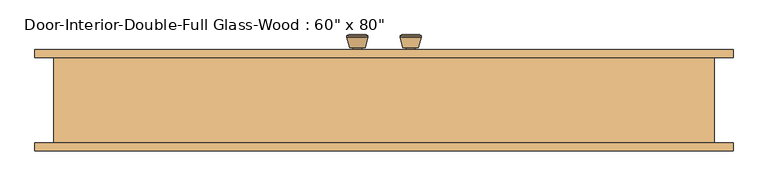
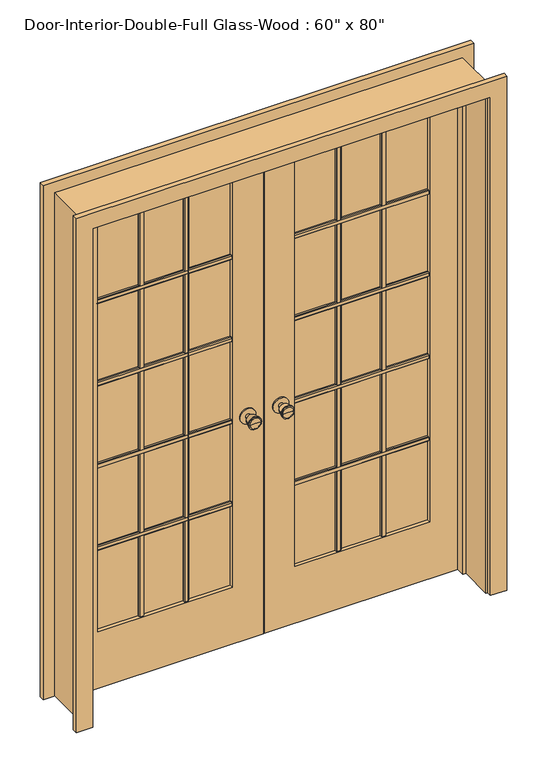
"""IFC4 building model written with IfcOpenShell, lengths in millimetres: door geometry."""

from ifc_helpers import new_model, si_unit, point, frame, frame_2d, origin, place, context, project, spatial, polyline, circle_curve, trimmed, segment, composite_curve, outline, extrude, faceted_brep, source, transform, mapped, element, save
from ifc_brep_helpers import plane_surface, cylinder_surface, revolved_surface, advanced_brep


def door_9d00318c(model_context):
    return source(origin(), model_context, "Body", "SolidModel", [
        advanced_brep(
        [(-63.5, 104.425, 914.4), (-73.5, 104.425, 914.4), (-53.5, 104.425, 914.4), (-83.9758676, 153.425, 914.4), (-63.5, 153.425, 914.4), (-43.0241324, 153.425, 914.4), (-88.5, 151.5971319, 914.4), (-38.5, 151.5971319, 914.4), (-88.5, 148.1334537, 914.4), (-38.5, 148.1334537, 914.4), (-82.136236, 123.425, 914.4), (-44.863764, 123.425, 914.4), (-73.5, 123.425, 914.4), (-53.5, 123.425, 914.4)],
        [
            (0, 1),
            (1, 2, circle_curve(frame((-63.5, 104.425, 914.4), z_axis=(0.0, -1.0, 0.0), x_axis=(1.0, 0.0, 0.0)), 10.0)),
            (2, 0),
            (2, 1, circle_curve(frame((-63.5, 104.425, 914.4), z_axis=(0.0, -1.0, 0.0), x_axis=(1.0, 0.0, 0.0)), 10.0)),
            (3, 4),
            (4, 5),
            (5, 3, circle_curve(frame((-63.5, 153.425, 914.4), z_axis=(0.0, 1.0, 0.0), x_axis=(1.0, 0.0, 0.0)), 20.4758676)),
            (3, 5, circle_curve(frame((-63.5, 153.425, 914.4), z_axis=(0.0, 1.0, 0.0), x_axis=(1.0, 0.0, 0.0)), 20.4758676)),
            (6, 3),
            (5, 7),
            (7, 6, circle_curve(frame((-63.5, 151.5971319, 914.4), z_axis=(0.0, 1.0, 0.0), x_axis=(1.0, 0.0, 0.0)), 25.0)),
            (6, 7, circle_curve(frame((-63.5, 151.5971319, 914.4), z_axis=(0.0, 1.0, 0.0), x_axis=(1.0, 0.0, 0.0)), 25.0)),
            (8, 6),
            (7, 9),
            (9, 8, circle_curve(frame((-63.5, 148.1334537, 914.4), z_axis=(0.0, 1.0, 0.0), x_axis=(1.0, 0.0, 0.0)), 25.0)),
            (8, 9, circle_curve(frame((-63.5, 148.1334537, 914.4), z_axis=(0.0, 1.0, 0.0), x_axis=(1.0, 0.0, 0.0)), 25.0)),
            (10, 8),
            (9, 11),
            (11, 10, circle_curve(frame((-63.5, 123.425, 914.4), z_axis=(0.0, 1.0, 0.0), x_axis=(1.0, 0.0, 0.0)), 18.636236)),
            (10, 11, circle_curve(frame((-63.5, 123.425, 914.4), z_axis=(0.0, 1.0, 0.0), x_axis=(1.0, 0.0, 0.0)), 18.636236)),
            (12, 10),
            (11, 13),
            (13, 12, circle_curve(frame((-63.5, 123.425, 914.4), z_axis=(0.0, 1.0, 0.0), x_axis=(1.0, 0.0, 0.0)), 10.0)),
            (12, 13, circle_curve(frame((-63.5, 123.425, 914.4), z_axis=(0.0, 1.0, 0.0), x_axis=(1.0, 0.0, 0.0)), 10.0)),
            (1, 12),
            (13, 2),
        ],
        [
            plane_surface(frame((-63.5, 104.425, 914.4), z_axis=(0.0, -1.0, 0.0), x_axis=(1.0, 0.0, 0.0))),
            plane_surface(frame((-63.5, 153.425, 914.4), z_axis=(0.0, 1.0, 0.0), x_axis=(1.0, 0.0, 0.0))),
            revolved_surface(polyline([(-43.0241324, 153.425, 914.4), (-38.5, 151.5971319, 914.4)]), (-63.5, 104.425, 914.4), (0.0, -1.0, 0.0)),
            cylinder_surface(frame((-63.5, 104.425, 914.4), z_axis=(0.0, -1.0, 0.0), x_axis=(1.0, 0.0, 0.0)), 25.0),
            revolved_surface(polyline([(-38.5, 148.1334537, 914.4), (-44.863764, 123.425, 914.4)]), (-63.5, 104.425, 914.4), (0.0, -1.0, 0.0)),
            plane_surface(frame((-63.5, 123.425, 914.4), z_axis=(0.0, -1.0, 0.0), x_axis=(1.0, 0.0, 0.0))),
            cylinder_surface(frame((-63.5, 104.425, 914.4), z_axis=(0.0, -1.0, 0.0), x_axis=(1.0, 0.0, 0.0)), 10.0),
        ],
        [
            (0, [[1, 2, 3]]),
            (0, [[-3, 4, -1]]),
            (1, [[5, 6, 7]]),
            (1, [[-6, -5, 8]]),
            (2, [[9, -7, 10, 11]]),
            (2, [[-10, -8, -9, 12]]),
            (3, [[13, -11, 14, 15]]),
            (3, [[-14, -12, -13, 16]]),
            (4, [[17, -15, 18, 19]]),
            (4, [[-18, -16, -17, 20]]),
            (5, [[21, -19, 22, 23]]),
            (5, [[-22, -20, -21, 24]]),
            (6, [[25, -23, 26, -2]]),
            (6, [[-26, -24, -25, -4]]),
        ],
    ),
        extrude(outline(composite_curve([segment(trimmed(circle_curve(frame_2d((914.4, -63.5)), 30.0), [point((914.4, -33.5))], [point((914.4, -93.5))], False, "CARTESIAN"), True, "CONTINUOUS"), segment(trimmed(circle_curve(frame_2d((914.4, -63.5)), 30.0), [point((914.4, -93.5))], [point((914.4, -33.5))], False, "CARTESIAN"), True, "CONTINUOUS")], self_intersect=False)), frame((0.0, 98.425, 0.0), z_axis=(0.0, 1.0, 0.0), x_axis=(0.0, 0.0, 1.0)), (0.0, 0.0, 1.0), 6.0),
        advanced_brep(
        [(-63.5, 57.5, 914.4), (-53.5, 57.5, 914.4), (-73.5, 57.5, 914.4), (-83.9758676, 8.5, 914.4), (-43.0241324, 8.5, 914.4), (-63.5, 8.5, 914.4), (-88.5, 10.3278681, 914.4), (-38.5, 10.3278681, 914.4), (-88.5, 13.7915463, 914.4), (-38.5, 13.7915463, 914.4), (-82.136236, 38.5, 914.4), (-44.863764, 38.5, 914.4), (-73.5, 38.5, 914.4), (-53.5, 38.5, 914.4)],
        [
            (0, 1),
            (1, 2, circle_curve(frame((-63.5, 57.5, 914.4), z_axis=(0.0, 1.0, 0.0), x_axis=(1.0, 0.0, 0.0)), 10.0)),
            (2, 0),
            (2, 1, circle_curve(frame((-63.5, 57.5, 914.4), z_axis=(0.0, 1.0, 0.0), x_axis=(1.0, 0.0, 0.0)), 10.0)),
            (3, 4, circle_curve(frame((-63.5, 8.5, 914.4), z_axis=(0.0, -1.0, 0.0), x_axis=(1.0, 0.0, 0.0)), 20.4758676)),
            (4, 5),
            (5, 3),
            (4, 3, circle_curve(frame((-63.5, 8.5, 914.4), z_axis=(0.0, -1.0, 0.0), x_axis=(1.0, 0.0, 0.0)), 20.4758676)),
            (6, 7, circle_curve(frame((-63.5, 10.3278681, 914.4), z_axis=(0.0, -1.0, 0.0), x_axis=(1.0, 0.0, 0.0)), 25.0)),
            (7, 4),
            (3, 6),
            (7, 6, circle_curve(frame((-63.5, 10.3278681, 914.4), z_axis=(0.0, -1.0, 0.0), x_axis=(1.0, 0.0, 0.0)), 25.0)),
            (8, 9, circle_curve(frame((-63.5, 13.7915463, 914.4), z_axis=(0.0, -1.0, 0.0), x_axis=(1.0, 0.0, 0.0)), 25.0)),
            (9, 7),
            (6, 8),
            (9, 8, circle_curve(frame((-63.5, 13.7915463, 914.4), z_axis=(0.0, -1.0, 0.0), x_axis=(1.0, 0.0, 0.0)), 25.0)),
            (10, 11, circle_curve(frame((-63.5, 38.5, 914.4), z_axis=(0.0, -1.0, 0.0), x_axis=(1.0, 0.0, 0.0)), 18.636236)),
            (11, 9),
            (8, 10),
            (11, 10, circle_curve(frame((-63.5, 38.5, 914.4), z_axis=(0.0, -1.0, 0.0), x_axis=(1.0, 0.0, 0.0)), 18.636236)),
            (12, 13, circle_curve(frame((-63.5, 38.5, 914.4), z_axis=(0.0, -1.0, 0.0), x_axis=(1.0, 0.0, 0.0)), 10.0)),
            (13, 11),
            (10, 12),
            (13, 12, circle_curve(frame((-63.5, 38.5, 914.4), z_axis=(0.0, -1.0, 0.0), x_axis=(1.0, 0.0, 0.0)), 10.0)),
            (1, 13),
            (12, 2),
        ],
        [
            plane_surface(frame((-63.5, 57.5, 914.4), z_axis=(0.0, 1.0, 0.0), x_axis=(1.0, 0.0, 0.0))),
            plane_surface(frame((-63.5, 8.5, 914.4), z_axis=(0.0, -1.0, 0.0), x_axis=(1.0, 0.0, 0.0))),
            revolved_surface(polyline([(-43.0241324, 8.5, 914.4), (-38.5, 10.3278681, 914.4)]), (-63.5, 57.5, 914.4), (0.0, 1.0, 0.0)),
            cylinder_surface(frame((-63.5, 57.5, 914.4), z_axis=(0.0, 1.0, 0.0), x_axis=(1.0, 0.0, 0.0)), 25.0),
            revolved_surface(polyline([(-38.5, 13.7915463, 914.4), (-44.863764, 38.5, 914.4)]), (-63.5, 57.5, 914.4), (0.0, 1.0, 0.0)),
            plane_surface(frame((-63.5, 38.5, 914.4), z_axis=(0.0, 1.0, 0.0), x_axis=(1.0, 0.0, 0.0))),
            cylinder_surface(frame((-63.5, 57.5, 914.4), z_axis=(0.0, 1.0, 0.0), x_axis=(1.0, 0.0, 0.0)), 10.0),
        ],
        [
            (0, [[1, 2, 3]]),
            (0, [[-3, 4, -1]]),
            (1, [[5, 6, 7]]),
            (1, [[8, -7, -6]]),
            (2, [[9, 10, -5, 11]]),
            (2, [[12, -11, -8, -10]]),
            (3, [[13, 14, -9, 15]]),
            (3, [[16, -15, -12, -14]]),
            (4, [[17, 18, -13, 19]]),
            (4, [[20, -19, -16, -18]]),
            (5, [[21, 22, -17, 23]]),
            (5, [[24, -23, -20, -22]]),
            (6, [[-2, 25, -21, 26]]),
            (6, [[-4, -26, -24, -25]]),
        ],
    ),
        extrude(outline(composite_curve([segment(trimmed(circle_curve(frame_2d((914.4, -63.5)), 30.0), [point((914.4, -33.5))], [point((914.4, -93.5))], False, "CARTESIAN"), True, "CONTINUOUS"), segment(trimmed(circle_curve(frame_2d((914.4, -63.5)), 30.0), [point((914.4, -93.5))], [point((914.4, -33.5))], False, "CARTESIAN"), True, "CONTINUOUS")], self_intersect=False)), frame((0.0, 57.5, 0.0), z_axis=(0.0, 1.0, 0.0), x_axis=(0.0, 0.0, 1.0)), (0.0, 0.0, 1.0), 6.0),
        extrude(outline(polyline([(77.47, 1586.23), (77.47, 1567.18), (71.12, 1567.18), (67.945, 1570.355), (67.945, 1583.055), (71.12, 1586.23), (77.47, 1586.23)])), frame((120.65, 0.0, 0.0), z_axis=(1.0, 0.0, 0.0), x_axis=(0.0, 1.0, 0.0)), (0.0, 0.0, 1.0), 520.7),
        extrude(outline(polyline([(77.47, 1249.9975), (77.47, 1230.9475), (71.12, 1230.9475), (67.945, 1234.1225), (67.945, 1246.8225), (71.12, 1249.9975), (77.47, 1249.9975)])), frame((120.65, 0.0, 0.0), z_axis=(1.0, 0.0, 0.0), x_axis=(0.0, 1.0, 0.0)), (0.0, 0.0, 1.0), 520.7),
        extrude(outline(polyline([(77.47, 913.765), (77.47, 894.715), (71.12, 894.715), (67.945, 897.89), (67.945, 910.59), (71.12, 913.765), (77.47, 913.765)])), frame((120.65, 0.0, 0.0), z_axis=(1.0, 0.0, 0.0), x_axis=(0.0, 1.0, 0.0)), (0.0, 0.0, 1.0), 520.7),
        extrude(outline(polyline([(77.47, 577.5325), (77.47, 558.4825), (71.12, 558.4825), (67.945, 561.6575), (67.945, 574.3575), (71.12, 577.5325), (77.47, 577.5325)])), frame((120.65, 0.0, 0.0), z_axis=(1.0, 0.0, 0.0), x_axis=(0.0, 1.0, 0.0)), (0.0, 0.0, 1.0), 520.7),
        extrude(outline(polyline([(458.2583333, 77.47), (477.3083333, 77.47), (477.3083333, 71.12), (474.1333333, 67.945), (461.4333333, 67.945), (458.2583333, 71.12), (458.2583333, 77.47)])), frame((0.0, 0.0, 231.775), z_axis=(0.0, 0.0, 1.0), x_axis=(1.0, 0.0, 0.0)), (0.0, 0.0, 1.0), 1681.1625),
        extrude(outline(polyline([(284.6916667, 77.47), (303.7416667, 77.47), (303.7416667, 71.12), (300.5666667, 67.945), (287.8666667, 67.945), (284.6916667, 71.12), (284.6916667, 77.47)])), frame((0.0, 0.0, 231.775), z_axis=(0.0, 0.0, 1.0), x_axis=(1.0, 0.0, 0.0)), (0.0, 0.0, 1.0), 1681.1625),
        extrude(outline(polyline([(84.455, 1586.23), (90.805, 1586.23), (93.98, 1583.055), (93.98, 1570.355), (90.805, 1567.18), (84.455, 1567.18), (84.455, 1586.23)])), frame((-641.35, 0.0, 0.0), z_axis=(1.0, 0.0, 0.0), x_axis=(0.0, 1.0, 0.0)), (0.0, 0.0, 1.0), 520.7),
        extrude(outline(polyline([(84.455, 1249.9975), (90.805, 1249.9975), (93.98, 1246.8225), (93.98, 1234.1225), (90.805, 1230.9475), (84.455, 1230.9475), (84.455, 1249.9975)])), frame((-641.35, 0.0, 0.0), z_axis=(1.0, 0.0, 0.0), x_axis=(0.0, 1.0, 0.0)), (0.0, 0.0, 1.0), 520.7),
        extrude(outline(polyline([(84.455, 913.765), (90.805, 913.765), (93.98, 910.59), (93.98, 897.89), (90.805, 894.715), (84.455, 894.715), (84.455, 913.765)])), frame((-641.35, 0.0, 0.0), z_axis=(1.0, 0.0, 0.0), x_axis=(0.0, 1.0, 0.0)), (0.0, 0.0, 1.0), 520.7),
        extrude(outline(polyline([(84.455, 577.5325), (90.805, 577.5325), (93.98, 574.3575), (93.98, 561.6575), (90.805, 558.4825), (84.455, 558.4825), (84.455, 577.5325)])), frame((-641.35, 0.0, 0.0), z_axis=(1.0, 0.0, 0.0), x_axis=(0.0, 1.0, 0.0)), (0.0, 0.0, 1.0), 520.7),
        extrude(outline(polyline([(-303.7416667, 84.455), (-303.7416667, 90.805), (-300.5666667, 93.98), (-287.8666667, 93.98), (-284.6916667, 90.805), (-284.6916667, 84.455), (-303.7416667, 84.455)])), frame((0.0, 0.0, 231.775), z_axis=(0.0, 0.0, 1.0), x_axis=(1.0, 0.0, 0.0)), (0.0, 0.0, 1.0), 1681.1625),
        extrude(outline(polyline([(-477.3083333, 84.455), (-477.3083333, 90.805), (-474.1333333, 93.98), (-461.4333333, 93.98), (-458.2583333, 90.805), (-458.2583333, 84.455), (-477.3083333, 84.455)])), frame((0.0, 0.0, 231.775), z_axis=(0.0, 0.0, 1.0), x_axis=(1.0, 0.0, 0.0)), (0.0, 0.0, 1.0), 1681.1625),
        extrude(outline(polyline([(84.455, 1586.23), (90.805, 1586.23), (93.98, 1583.055), (93.98, 1570.355), (90.805, 1567.18), (84.455, 1567.18), (84.455, 1586.23)])), frame((120.65, 0.0, 0.0), z_axis=(1.0, 0.0, 0.0), x_axis=(0.0, 1.0, 0.0)), (0.0, 0.0, 1.0), 520.7),
        extrude(outline(polyline([(84.455, 1249.9975), (90.805, 1249.9975), (93.98, 1246.8225), (93.98, 1234.1225), (90.805, 1230.9475), (84.455, 1230.9475), (84.455, 1249.9975)])), frame((120.65, 0.0, 0.0), z_axis=(1.0, 0.0, 0.0), x_axis=(0.0, 1.0, 0.0)), (0.0, 0.0, 1.0), 520.7),
        extrude(outline(polyline([(84.455, 913.765), (90.805, 913.765), (93.98, 910.59), (93.98, 897.89), (90.805, 894.715), (84.455, 894.715), (84.455, 913.765)])), frame((120.65, 0.0, 0.0), z_axis=(1.0, 0.0, 0.0), x_axis=(0.0, 1.0, 0.0)), (0.0, 0.0, 1.0), 520.7),
        extrude(outline(polyline([(84.455, 577.5325), (90.805, 577.5325), (93.98, 574.3575), (93.98, 561.6575), (90.805, 558.4825), (84.455, 558.4825), (84.455, 577.5325)])), frame((120.65, 0.0, 0.0), z_axis=(1.0, 0.0, 0.0), x_axis=(0.0, 1.0, 0.0)), (0.0, 0.0, 1.0), 520.7),
        extrude(outline(polyline([(458.2583333, 84.455), (458.2583333, 90.805), (461.4333333, 93.98), (474.1333333, 93.98), (477.3083333, 90.805), (477.3083333, 84.455), (458.2583333, 84.455)])), frame((0.0, 0.0, 231.775), z_axis=(0.0, 0.0, 1.0), x_axis=(1.0, 0.0, 0.0)), (0.0, 0.0, 1.0), 1681.1625),
        extrude(outline(polyline([(284.6916667, 84.455), (284.6916667, 90.805), (287.8666667, 93.98), (300.5666667, 93.98), (303.7416667, 90.805), (303.7416667, 84.455), (284.6916667, 84.455)])), frame((0.0, 0.0, 231.775), z_axis=(0.0, 0.0, 1.0), x_axis=(1.0, 0.0, 0.0)), (0.0, 0.0, 1.0), 1681.1625),
        extrude(outline(polyline([(77.47, 1586.23), (77.47, 1567.18), (71.12, 1567.18), (67.945, 1570.355), (67.945, 1583.055), (71.12, 1586.23), (77.47, 1586.23)])), frame((-641.35, 0.0, 0.0), z_axis=(1.0, 0.0, 0.0), x_axis=(0.0, 1.0, 0.0)), (0.0, 0.0, 1.0), 520.7),
        extrude(outline(polyline([(77.47, 1249.9975), (77.47, 1230.9475), (71.12, 1230.9475), (67.945, 1234.1225), (67.945, 1246.8225), (71.12, 1249.9975), (77.47, 1249.9975)])), frame((-641.35, 0.0, 0.0), z_axis=(1.0, 0.0, 0.0), x_axis=(0.0, 1.0, 0.0)), (0.0, 0.0, 1.0), 520.7),
        extrude(outline(polyline([(77.47, 913.765), (77.47, 894.715), (71.12, 894.715), (67.945, 897.89), (67.945, 910.59), (71.12, 913.765), (77.47, 913.765)])), frame((-641.35, 0.0, 0.0), z_axis=(1.0, 0.0, 0.0), x_axis=(0.0, 1.0, 0.0)), (0.0, 0.0, 1.0), 520.7),
        extrude(outline(polyline([(77.47, 577.5325), (77.47, 558.4825), (71.12, 558.4825), (67.945, 561.6575), (67.945, 574.3575), (71.12, 577.5325), (77.47, 577.5325)])), frame((-641.35, 0.0, 0.0), z_axis=(1.0, 0.0, 0.0), x_axis=(0.0, 1.0, 0.0)), (0.0, 0.0, 1.0), 520.7),
        extrude(outline(polyline([(-303.7416667, 77.47), (-284.6916667, 77.47), (-284.6916667, 71.12), (-287.8666667, 67.945), (-300.5666667, 67.945), (-303.7416667, 71.12), (-303.7416667, 77.47)])), frame((0.0, 0.0, 231.775), z_axis=(0.0, 0.0, 1.0), x_axis=(1.0, 0.0, 0.0)), (0.0, 0.0, 1.0), 1681.1625),
        extrude(outline(polyline([(-477.3083333, 77.47), (-458.2583333, 77.47), (-458.2583333, 71.12), (-461.4333333, 67.945), (-474.1333333, 67.945), (-477.3083333, 71.12), (-477.3083333, 77.47)])), frame((0.0, 0.0, 231.775), z_axis=(0.0, 0.0, 1.0), x_axis=(1.0, 0.0, 0.0)), (0.0, 0.0, 1.0), 1681.1625),
        advanced_brep(
        [(63.5, 57.5, 914.4), (73.5, 57.5, 914.4), (53.5, 57.5, 914.4), (83.9758676, 8.5, 914.4), (63.5, 8.5, 914.4), (43.0241324, 8.5, 914.4), (88.5, 10.3278681, 914.4), (38.5, 10.3278681, 914.4), (88.5, 13.7915463, 914.4), (38.5, 13.7915463, 914.4), (82.136236, 38.5, 914.4), (44.863764, 38.5, 914.4), (73.5, 38.5, 914.4), (53.5, 38.5, 914.4)],
        [
            (0, 1),
            (1, 2, circle_curve(frame((63.5, 57.5, 914.4), z_axis=(0.0, 1.0, 0.0), x_axis=(-1.0, 0.0, 0.0)), 10.0)),
            (2, 0),
            (2, 1, circle_curve(frame((63.5, 57.5, 914.4), z_axis=(0.0, 1.0, 0.0), x_axis=(-1.0, 0.0, 0.0)), 10.0)),
            (3, 4),
            (4, 5),
            (5, 3, circle_curve(frame((63.5, 8.5, 914.4), z_axis=(0.0, -1.0, 0.0), x_axis=(-1.0, 0.0, 0.0)), 20.4758676)),
            (3, 5, circle_curve(frame((63.5, 8.5, 914.4), z_axis=(0.0, -1.0, 0.0), x_axis=(-1.0, 0.0, 0.0)), 20.4758676)),
            (6, 3),
            (5, 7),
            (7, 6, circle_curve(frame((63.5, 10.3278681, 914.4), z_axis=(0.0, -1.0, 0.0), x_axis=(-1.0, 0.0, 0.0)), 25.0)),
            (6, 7, circle_curve(frame((63.5, 10.3278681, 914.4), z_axis=(0.0, -1.0, 0.0), x_axis=(-1.0, 0.0, 0.0)), 25.0)),
            (8, 6),
            (7, 9),
            (9, 8, circle_curve(frame((63.5, 13.7915463, 914.4), z_axis=(0.0, -1.0, 0.0), x_axis=(-1.0, 0.0, 0.0)), 25.0)),
            (8, 9, circle_curve(frame((63.5, 13.7915463, 914.4), z_axis=(0.0, -1.0, 0.0), x_axis=(-1.0, 0.0, 0.0)), 25.0)),
            (10, 8),
            (9, 11),
            (11, 10, circle_curve(frame((63.5, 38.5, 914.4), z_axis=(0.0, -1.0, 0.0), x_axis=(-1.0, 0.0, 0.0)), 18.636236)),
            (10, 11, circle_curve(frame((63.5, 38.5, 914.4), z_axis=(0.0, -1.0, 0.0), x_axis=(-1.0, 0.0, 0.0)), 18.636236)),
            (12, 10),
            (11, 13),
            (13, 12, circle_curve(frame((63.5, 38.5, 914.4), z_axis=(0.0, -1.0, 0.0), x_axis=(-1.0, 0.0, 0.0)), 10.0)),
            (12, 13, circle_curve(frame((63.5, 38.5, 914.4), z_axis=(0.0, -1.0, 0.0), x_axis=(-1.0, 0.0, 0.0)), 10.0)),
            (1, 12),
            (13, 2),
        ],
        [
            plane_surface(frame((63.5, 57.5, 914.4), z_axis=(0.0, 1.0, 0.0), x_axis=(-1.0, 0.0, 0.0))),
            plane_surface(frame((63.5, 8.5, 914.4), z_axis=(0.0, -1.0, 0.0), x_axis=(-1.0, 0.0, 0.0))),
            revolved_surface(polyline([(43.0241324, 8.5, 914.4), (38.5, 10.3278681, 914.4)]), (63.5, 57.5, 914.4), (0.0, 1.0, 0.0)),
            cylinder_surface(frame((63.5, 57.5, 914.4), z_axis=(0.0, 1.0, 0.0), x_axis=(-1.0, 0.0, 0.0)), 25.0),
            revolved_surface(polyline([(38.5, 13.7915463, 914.4), (44.863764, 38.5, 914.4)]), (63.5, 57.5, 914.4), (0.0, 1.0, 0.0)),
            plane_surface(frame((63.5, 38.5, 914.4), z_axis=(0.0, 1.0, 0.0), x_axis=(-1.0, 0.0, 0.0))),
            cylinder_surface(frame((63.5, 57.5, 914.4), z_axis=(0.0, 1.0, 0.0), x_axis=(-1.0, 0.0, 0.0)), 10.0),
        ],
        [
            (0, [[1, 2, 3]]),
            (0, [[-3, 4, -1]]),
            (1, [[5, 6, 7]]),
            (1, [[-6, -5, 8]]),
            (2, [[9, -7, 10, 11]]),
            (2, [[-10, -8, -9, 12]]),
            (3, [[13, -11, 14, 15]]),
            (3, [[-14, -12, -13, 16]]),
            (4, [[17, -15, 18, 19]]),
            (4, [[-18, -16, -17, 20]]),
            (5, [[21, -19, 22, 23]]),
            (5, [[-22, -20, -21, 24]]),
            (6, [[25, -23, 26, -2]]),
            (6, [[-26, -24, -25, -4]]),
        ],
    ),
        extrude(outline(composite_curve([segment(trimmed(circle_curve(frame_2d((914.4, 63.5)), 30.0), [point((914.4, 33.5))], [point((914.4, 93.5))], False, "CARTESIAN"), True, "CONTINUOUS"), segment(trimmed(circle_curve(frame_2d((914.4, 63.5)), 30.0), [point((914.4, 93.5))], [point((914.4, 33.5))], False, "CARTESIAN"), True, "CONTINUOUS")], self_intersect=False)), frame((0.0, 57.5, 0.0), z_axis=(0.0, 1.0, 0.0), x_axis=(0.0, 0.0, 1.0)), (0.0, 0.0, 1.0), 6.0),
        advanced_brep(
        [(63.5, 104.425, 914.4), (53.5, 104.425, 914.4), (73.5, 104.425, 914.4), (83.9758676, 153.425, 914.4), (43.0241324, 153.425, 914.4), (63.5, 153.425, 914.4), (88.5, 151.5971319, 914.4), (38.5, 151.5971319, 914.4), (88.5, 148.1334537, 914.4), (38.5, 148.1334537, 914.4), (82.136236, 123.425, 914.4), (44.863764, 123.425, 914.4), (73.5, 123.425, 914.4), (53.5, 123.425, 914.4)],
        [
            (0, 1),
            (1, 2, circle_curve(frame((63.5, 104.425, 914.4), z_axis=(0.0, -1.0, 0.0), x_axis=(-1.0, 0.0, 0.0)), 10.0)),
            (2, 0),
            (2, 1, circle_curve(frame((63.5, 104.425, 914.4), z_axis=(0.0, -1.0, 0.0), x_axis=(-1.0, 0.0, 0.0)), 10.0)),
            (3, 4, circle_curve(frame((63.5, 153.425, 914.4), z_axis=(0.0, 1.0, 0.0), x_axis=(-1.0, 0.0, 0.0)), 20.4758676)),
            (4, 5),
            (5, 3),
            (4, 3, circle_curve(frame((63.5, 153.425, 914.4), z_axis=(0.0, 1.0, 0.0), x_axis=(-1.0, 0.0, 0.0)), 20.4758676)),
            (6, 7, circle_curve(frame((63.5, 151.5971319, 914.4), z_axis=(0.0, 1.0, 0.0), x_axis=(-1.0, 0.0, 0.0)), 25.0)),
            (7, 4),
            (3, 6),
            (7, 6, circle_curve(frame((63.5, 151.5971319, 914.4), z_axis=(0.0, 1.0, 0.0), x_axis=(-1.0, 0.0, 0.0)), 25.0)),
            (8, 9, circle_curve(frame((63.5, 148.1334537, 914.4), z_axis=(0.0, 1.0, 0.0), x_axis=(-1.0, 0.0, 0.0)), 25.0)),
            (9, 7),
            (6, 8),
            (9, 8, circle_curve(frame((63.5, 148.1334537, 914.4), z_axis=(0.0, 1.0, 0.0), x_axis=(-1.0, 0.0, 0.0)), 25.0)),
            (10, 11, circle_curve(frame((63.5, 123.425, 914.4), z_axis=(0.0, 1.0, 0.0), x_axis=(-1.0, 0.0, 0.0)), 18.636236)),
            (11, 9),
            (8, 10),
            (11, 10, circle_curve(frame((63.5, 123.425, 914.4), z_axis=(0.0, 1.0, 0.0), x_axis=(-1.0, 0.0, 0.0)), 18.636236)),
            (12, 13, circle_curve(frame((63.5, 123.425, 914.4), z_axis=(0.0, 1.0, 0.0), x_axis=(-1.0, 0.0, 0.0)), 10.0)),
            (13, 11),
            (10, 12),
            (13, 12, circle_curve(frame((63.5, 123.425, 914.4), z_axis=(0.0, 1.0, 0.0), x_axis=(-1.0, 0.0, 0.0)), 10.0)),
            (1, 13),
            (12, 2),
        ],
        [
            plane_surface(frame((63.5, 104.425, 914.4), z_axis=(0.0, -1.0, 0.0), x_axis=(-1.0, 0.0, 0.0))),
            plane_surface(frame((63.5, 153.425, 914.4), z_axis=(0.0, 1.0, 0.0), x_axis=(-1.0, 0.0, 0.0))),
            revolved_surface(polyline([(43.0241324, 153.425, 914.4), (38.5, 151.5971319, 914.4)]), (63.5, 104.425, 914.4), (0.0, -1.0, 0.0)),
            cylinder_surface(frame((63.5, 104.425, 914.4), z_axis=(0.0, -1.0, 0.0), x_axis=(-1.0, 0.0, 0.0)), 25.0),
            revolved_surface(polyline([(38.5, 148.1334537, 914.4), (44.863764, 123.425, 914.4)]), (63.5, 104.425, 914.4), (0.0, -1.0, 0.0)),
            plane_surface(frame((63.5, 123.425, 914.4), z_axis=(0.0, -1.0, 0.0), x_axis=(-1.0, 0.0, 0.0))),
            cylinder_surface(frame((63.5, 104.425, 914.4), z_axis=(0.0, -1.0, 0.0), x_axis=(-1.0, 0.0, 0.0)), 10.0),
        ],
        [
            (0, [[1, 2, 3]]),
            (0, [[-3, 4, -1]]),
            (1, [[5, 6, 7]]),
            (1, [[8, -7, -6]]),
            (2, [[9, 10, -5, 11]]),
            (2, [[12, -11, -8, -10]]),
            (3, [[13, 14, -9, 15]]),
            (3, [[16, -15, -12, -14]]),
            (4, [[17, 18, -13, 19]]),
            (4, [[20, -19, -16, -18]]),
            (5, [[21, 22, -17, 23]]),
            (5, [[24, -23, -20, -22]]),
            (6, [[-2, 25, -21, 26]]),
            (6, [[-4, -26, -24, -25]]),
        ],
    ),
        extrude(outline(composite_curve([segment(trimmed(circle_curve(frame_2d((914.4, 63.5)), 30.0), [point((914.4, 33.5))], [point((914.4, 93.5))], False, "CARTESIAN"), True, "CONTINUOUS"), segment(trimmed(circle_curve(frame_2d((914.4, 63.5)), 30.0), [point((914.4, 93.5))], [point((914.4, 33.5))], False, "CARTESIAN"), True, "CONTINUOUS")], self_intersect=False)), frame((0.0, 98.425, 0.0), z_axis=(0.0, 1.0, 0.0), x_axis=(0.0, 0.0, 1.0)), (0.0, 0.0, 1.0), 6.0),
        extrude(outline(polyline([(0.0, 768.35), (0.0, 831.85), (2101.85, 831.85), (2101.85, -831.85), (0.0, -831.85), (0.0, -768.35), (2038.35, -768.35), (2038.35, 768.35), (0.0, 768.35)])), frame((0.0, 98.425, 0.0), z_axis=(0.0, 1.0, 0.0), x_axis=(0.0, 0.0, 1.0)), (0.0, 0.0, 1.0), 19.05),
        extrude(outline(polyline([(0.0, 768.35), (0.0, 831.85), (2101.85, 831.85), (2101.85, -831.85), (0.0, -831.85), (0.0, -768.35), (2038.35, -768.35), (2038.35, 768.35), (0.0, 768.35)])), frame((0.0, -123.825, 0.0), z_axis=(0.0, 1.0, 0.0), x_axis=(0.0, 0.0, 1.0)), (0.0, 0.0, 1.0), 19.05),
        extrude(outline(polyline([(2032.0, -762.0), (0.0, -762.0), (0.0, -1.6019111), (2032.0, -1.6019111), (2032.0, -762.0)]), holes=[polyline([(231.775, -641.35), (1912.9375, -641.35), (1912.9375, -120.65), (231.775, -120.65), (231.775, -641.35)])]), frame((0.0, 63.5, 0.0), z_axis=(0.0, 1.0, 0.0), x_axis=(0.0, 0.0, 1.0)), (0.0, 0.0, 1.0), 34.925),
        extrude(outline(polyline([(0.0, 762.0), (2032.0, 762.0), (2032.0, 1.5875), (0.0, 1.5875), (0.0, 762.0)]), holes=[polyline([(1912.9375, 120.65), (1912.9375, 641.35), (231.775, 641.35), (231.775, 120.65), (1912.9375, 120.65)])]), frame((0.0, 63.5, 0.0), z_axis=(0.0, 1.0, 0.0), x_axis=(0.0, 0.0, 1.0)), (0.0, 0.0, 1.0), 34.925),
        faceted_brep([(787.4, 98.425, 0.0), (787.4, -104.775, 0.0), (762.0, -104.775, 0.0), (762.0, 28.575, 0.0), (749.3, 28.575, 0.0), (749.3, 63.5, 0.0), (762.0, 63.5, 0.0), (762.0, 98.425, 0.0), (787.4, 98.425, 2057.4), (787.4, -104.775, 2057.4), (-787.4, -104.775, 2057.4), (-787.4, -104.775, 0.0), (-762.0, -104.775, 0.0), (-762.0, -104.775, 2032.0), (762.0, -104.775, 2032.0), (762.0, 28.575, 2032.0), (-762.0, 28.575, 2032.0), (-762.0, 28.575, 0.0), (-749.3, 28.575, 0.0), (-749.3, 28.575, 2019.3), (749.3, 28.575, 2019.3), (749.3, 63.5, 2019.3), (1.5875, 63.5, 2019.3), (-1.6019111, 63.5, 2019.3), (-749.3, 63.5, 2019.3), (-749.3, 63.5, 0.0), (-762.0, 63.5, 0.0), (-762.0, 63.5, 2032.0), (-1.6019111, 63.5, 2032.0), (1.5875, 63.5, 2032.0), (762.0, 63.5, 2032.0), (762.0, 98.425, 2032.0), (1.5875, 98.425, 2032.0), (-1.6019111, 98.425, 2032.0), (-762.0, 98.425, 2032.0), (-762.0, 98.425, 0.0), (-787.4, 98.425, 0.0), (-787.4, 98.425, 2057.4)], [[[0, 1, 2, 3, 4, 5, 6, 7]], [[1, 0, 8, 9]], [[2, 1, 9, 10, 11, 12, 13, 14]], [[3, 2, 14, 15]], [[4, 3, 15, 16, 17, 18, 19, 20]], [[5, 4, 20, 21]], [[6, 5, 21, 22, 23, 24, 25, 26, 27, 28, 29, 30]], [[7, 6, 30, 31]], [[0, 7, 31, 32, 33, 34, 35, 36, 37, 8]], [[9, 8, 37, 10]], [[14, 13, 16, 15]], [[20, 19, 24, 23, 22, 21]], [[31, 30, 29, 28, 27, 34, 33, 32]], [[12, 11, 36, 35, 26, 25, 18, 17]], [[11, 10, 37, 36]], [[13, 12, 17, 16]], [[19, 18, 25, 24]], [[27, 26, 35, 34]]]),
        extrude(outline(polyline([(641.35, 77.47), (120.65, 77.47), (120.65, 84.455), (641.35, 84.455), (641.35, 77.47)])), frame((0.0, 0.0, 231.775), z_axis=(0.0, 0.0, 1.0), x_axis=(1.0, 0.0, 0.0)), (0.0, 0.0, 1.0), 1681.1625),
        extrude(outline(polyline([(-120.65, 77.47), (-641.35, 77.47), (-641.35, 84.455), (-120.65, 84.455), (-120.65, 77.47)])), frame((0.0, 0.0, 231.775), z_axis=(0.0, 0.0, 1.0), x_axis=(1.0, 0.0, 0.0)), (0.0, 0.0, 1.0), 1681.1625),
    ])


if __name__ == "__main__":
    model = new_model("IFC4")
    model_context = context("Model", 3, world=origin())
    ifc_project = project(units=[si_unit("LENGTHUNIT", "METRE", prefix="MILLI")], contexts=[model_context])
    site = spatial("IfcSite", under=ifc_project)
    building = spatial("IfcBuilding", under=site)
    placement = place(None, origin())
    door_shape = door_9d00318c(model_context)
    element("IfcDoor", 1, ObjectType="Door-Interior-Double-Full Glass-Wood : 60\" x 80\"", at=placement, inside=building, context=model_context, shape_type="MappedRepresentation", body=[
        mapped(door_shape, transform((0.0, 0.0, 0.0), x_axis=(1.0, 0.0, 0.0), y_axis=(0.0, 1.0, 0.0), z_axis=(0.0, 0.0, 1.0))),
    ])
    save(model, "model.ifc")

# Revit data of these elements
# Type "Door-Interior-Double-Full Glass-Wood : 60\" x 80\""
#   Type Mark = "9"
#   Assembly Code = "C1020300"
#   Analytic Construction = "French door, wood frame with single glass"
#   Top Rail = 0' - 4 11/16"
#   Thickness = 0' - 1 3/8"
#   Thermal Resistance (R) = 1.0696 (h·ft²·°F)/BTU
#   Swing Angle [instance default] = 90.00°
#   Stiles = 0' - 4 3/4"
#   Rough Width = 5' - 2"
#   Rough Height = 6' - 9"
#   Panel Width = 2' - 6"
#   Height = 6' - 8"
#   Width = 5' - 0"
#   Heat Transfer Coefficient (U) = 0.9350 BTU/(h·ft²·°F)
#   Bottom Rail = 0' - 9 1/8"
#   Show Grill [instance default] = yes
#   Trim Material = Cherry
#   Panel Material = Cherry
#   Frame Material = Cherry
#   Door Handle Material = Aluminum
#   Visual Light Transmittance = 0
#   Solar Heat Gain Coefficient = 0
#   Wall Closure = (empty or 0)
#   Function = (empty or 0)
# Element 1 (IfcDoor, "Door-Interior-Double-Full Glass-Wood : 60\" x 80\"")
#   Materials on its faces: "Cherry", "Aluminum", "Glass"
# Materials
#   "Cherry": class "Wood", colour RGB 226 177 128, transparency 0, Description = "Prunus Serotina", Cost = 0
#   "Aluminum": class "Metal", colour RGB 247 247 247, transparency 0, Description = "Aluminum 6061", Cost = 0
#   "Glass": class "Glass", colour RGB 0 128 192, transparency 0.75, Description = "Soda Lime Glass", Cost = 0
